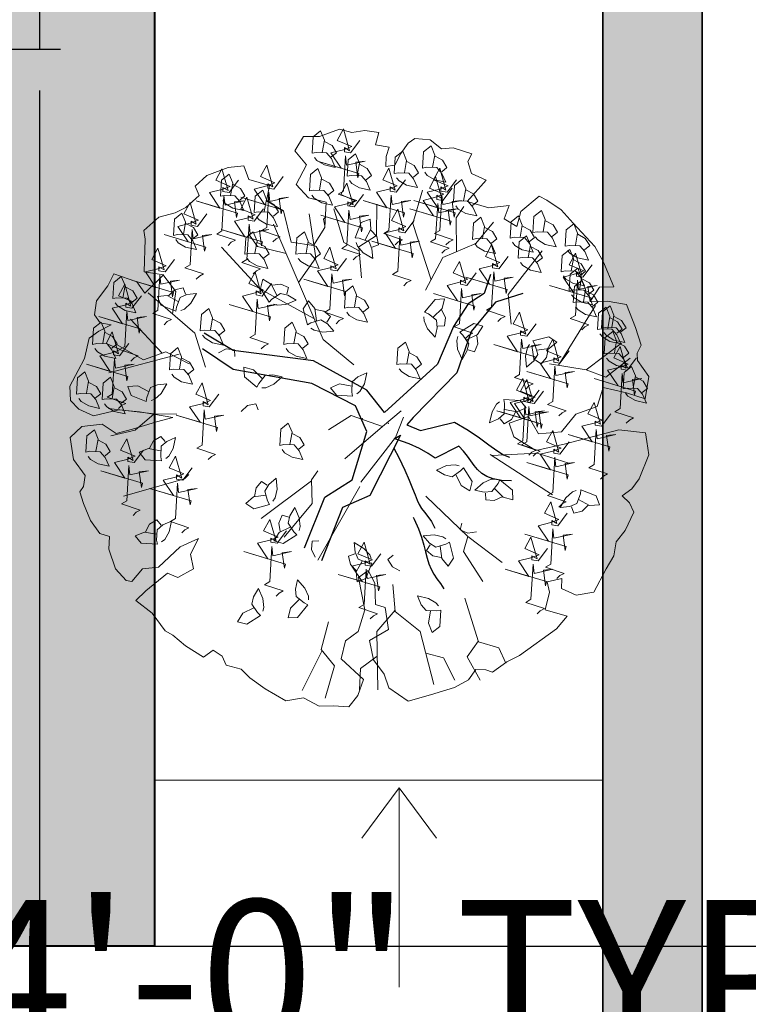
# Model space of a CAD drawing. Units: inches. Extents: x 2337 to 3570, y 1258 to 1938.
# Tile 25 of 30: x 3427 to 3471, y 1539 to 1598. Entities that reach past the tile are written whole.
import ezdxf

# ---------------------------------------------------------------- set-up
doc = ezdxf.new("R2010")
doc.units = ezdxf.units.IN
for name, color, linetype, lineweight in [('A-ANNO-DIMS', 2, 'Continuous', 18), ('A-ANNO-SYMB', 7, 'Continuous', 18), ('A-FLOR-STRS', 7, 'Continuous', 20), ('A-WALL', 7, 'Continuous', 40), ('ARBOL', 74, 'Continuous', 13), ('C-PROP', 7, 'Continuous', 35)]:
    doc.layers.add(name, color=color, linetype=linetype, lineweight=lineweight)
doc.layers.add('A-WALL-PATT', color=18, linetype='Continuous', lineweight=13, true_color=0x000000)
doc.layers.add('C-PROP-PATT', color=251, linetype='Continuous', lineweight=13, true_color=0x636466)
doc.layers.add('TALLO', color=36, linetype='Continuous')
doc.styles.get("Standard").update_dxf_attribs({"font": 'arial.ttf'})
doc.dimstyles.new('ISO-25', dxfattribs={"dimtxt": 9, "dimasz": 2.5, "dimexe": 1.25, "dimexo": 0.625, "dimtad": 1, "dimdec": 1, "dimlunit": 3, "dimtxsty": 'Standard', "dimcen": 2.5, "dimadec": 0, "dimazin": 0, "dimtfac": 1, "dimtdec": 1, "dimtmove": 0, "dimatfit": 3, "dimfxl": 1, "dimarcsym": 0})

# ---------------------------------------------------------------- blocks, each defined once
blk = doc.blocks.new('fresno')
at = {"layer": 'ARBOL'}
for p, q in [((2.96, 0.991), (3.575, 1.984)), ((-3.638, 1.194), (-4.164, 1.76)), ((-1.151, -0.932), (-1.99, -1.556)), ((-0.974, -3.757), (-1.31, -4.423))]:
    blk.add_line(p, q, dxfattribs=at)
blk.add_lwpolyline([(0.823, 4.745), (0.566, 4.764), (0.459, 4.687), (0.336, 4.518), (0.233, 4.322), (0.087, 4.298), (0.091, 4.464), (0.14, 4.621), (-0.09, 4.659), (-0.033, 4.863), (-0.264, 4.901), (-0.483, 4.866), (-0.686, 4.924), (-1.021, 4.801), (-1.288, 4.8), (-1.431, 4.563), (-1.234, 4.327), (-1.406, 4), (-1.205, 3.778), (-0.909, 3.705), (-0.931, 3.283), (-1.122, 2.983), (-1.491, 3.043), (-1.619, 3.562), (-1.9, 3.727), (-1.851, 3.982), (-2.197, 4.084), (-2.278, 4.31), (-2.543, 4.283), (-2.896, 4.152), (-3.091, 3.971), (-3.022, 3.817), (-3.244, 3.617), (-3.424, 3.528), (-3.697, 3.455), (-3.946, 3.236), (-3.922, 3.09), (-3.94, 2.548), (-3.617, 2.495), (-3.927, 2.19), (-4.062, 2.379), (-4.443, 2.512), (-4.546, 2.316), (-4.73, 2.062), (-4.767, 1.832), (-4.671, 1.698), (-4.486, 1.667), (-4.693, 1.559), (-4.854, 1.444), (-4.934, 1.102), (-5.037, 0.905), (-5.175, 0.644), (-5.166, 0.406), (-5.024, 0.264), (-4.781, 0.153), (-4.363, 0.249), (-4.014, 0.215), (-3.783, 0.177), (-3.46, 0.124), (-3.733, 0.051), (-4.132, -0.073), (-4.404, -0.146), (-4.639, 0.011), (-4.977, -0.028), (-5.172, -0.209), (-5.113, -0.574), (-4.921, -0.843), (-4.951, -1.027), (-5.012, -1.112), (-4.95, -1.311), (-4.83, -1.592), (-4.676, -1.807), (-4.518, -1.856), (-4.529, -2.068), (-4.417, -2.394), (-4.236, -2.59), (-4.143, -2.605), (-3.967, -2.397), (-3.703, -2.37), (-3.339, -2.027), (-3.032, -1.889), (-3.169, -2.15), (-3.115, -2.396), (-3.376, -2.542), (-3.552, -2.466), (-3.909, -2.762), (-4.077, -2.924), (-3.804, -3.135), (-3.592, -3.43), (-3.461, -3.499), (-3.253, -3.676), (-2.953, -3.867), (-2.792, -3.752), (-2.642, -3.848), (-2.572, -4.001), (-2.323, -4.066), (-2.18, -4.208), (-1.926, -4.392), (-1.58, -4.591), (-1.288, -4.545), (-1.027, -4.683), (-0.788, -4.675), (-0.531, -4.693), (-0.382, -4.505), (-0.29, -4.236), (-0.66, -3.891), (-0.588, -3.595), (-0.374, -3.441), (-0.267, -3.079), (-0.368, -2.541), (-0.208, -2.426), (-0.099, -2.633), (-0.087, -2.991), (0.071, -3.04), (0.129, -3.405), (-0.185, -3.59), (-0.119, -3.909), (0.055, -4.151), (0.136, -4.377), (0.456, -4.596), (0.828, -4.491), (1.227, -4.368), (1.461, -4.241), (1.583, -4.071), (1.748, -4.075), (1.86, -4.117), (2.101, -3.944), (2.308, -3.836), (2.925, -3.393), (3.101, -3.185), (2.74, -3.078), (2.812, -2.782), (2.769, -2.61), (3.015, -2.555), (3.012, -2.721), (3.254, -2.832), (3.546, -2.785), (3.752, -2.393), (3.882, -2.177), (3.92, -1.947), (4.069, -1.758), (4.214, -1.451), (4.144, -1.297), (4.021, -1.182), (4.182, -1.067), (4.304, -0.897), (4.464, -0.497), (4.429, -0.279), (4.406, -0.133), (3.964, -0.083), (3.074, -0.315), (2.582, -0.424), (2.217, -0.197), (2.136, 0.029), (2.462, 0.141), (2.628, -0.147), (3.012, -0.116), (3.249, 0.177), (3.602, 0.308), (3.701, 0.623), (4.089, 0.535), (4.404, 0.436), (4.464, 0.805), (4.272, 1.074), (4.267, 1.193), (4.336, 1.324), (4.243, 1.623), (4.092, 2.003), (3.769, 2.057), (3.485, 2.056), (3.642, 2.291), (3.88, 2.299), (3.71, 2.706), (3.563, 2.967), (3.201, 3.358), (3.001, 3.581), (2.766, 3.738), (2.635, 3.807), (2.332, 3.549), (2.268, 3.299), (2.052, 3.429), (2.136, 3.652), (1.798, 3.613), (1.437, 3.72), (1.755, 4.071), (1.513, 4.182), (1.451, 4.381), (1.519, 4.512), (1.204, 4.611), (1.012, 4.596)], close=True, dxfattribs=at)
for points in [[(-0.346, 4.735), (-0.501, 4.528), (-0.605, 4.545), (-0.605, 4.614), (-0.519, 4.563), (-0.622, 4.925), (-0.726, 4.735), (-0.484, 4.632), (-0.622, 4.58), (-0.829, 4.528), (-0.657, 4.27), (-1.053, 4.39), (-0.363, 4.183), (-0.381, 4.114), (-0.415, 4.373), (-0.26, 4.39), (-0.57, 4.321), (-0.588, 4.476), (-0.622, 3.89), (-0.708, 3.839), (-0.398, 3.735), (-0.467, 3.701), (-0.519, 3.649)], [(-1.104, 4.45), (-1.063, 4.399), (-0.939, 4.325), (-0.757, 4.285), (-0.82, 4.431), (-0.903, 4.527), (-1.075, 4.533), (-1.143, 4.521), (-1.126, 4.792), (-1.002, 4.891), (-0.939, 4.738), (-0.975, 4.535)], [(-0.935, 4.717), (-0.809, 4.65), (-0.736, 4.529), (-0.824, 4.459)], [(0.734, 4.203), (0.775, 4.152), (0.9, 4.078), (1.082, 4.038), (1.018, 4.185), (0.936, 4.281), (0.763, 4.287), (0.696, 4.274), (0.712, 4.546), (0.837, 4.645), (0.899, 4.491), (0.863, 4.289)], [(-0.521, 4.069), (-0.48, 4.018), (-0.356, 3.944), (-0.174, 3.904), (-0.237, 4.051), (-0.32, 4.146), (-0.492, 4.152), (-0.56, 4.14), (-0.543, 4.411), (-0.419, 4.511), (-0.356, 4.357), (-0.392, 4.154)], [(0.263, 4.114), (0.304, 4.063), (0.429, 3.989), (0.611, 3.948), (0.547, 4.095), (0.465, 4.191), (0.293, 4.197), (0.225, 4.185), (0.242, 4.456), (0.366, 4.555), (0.428, 4.402), (0.393, 4.199)], [(0.904, 4.471), (1.029, 4.404), (1.102, 4.282), (1.015, 4.212)], [(-2.368, 4.073), (-2.523, 3.866), (-2.627, 3.883), (-2.627, 3.952), (-2.541, 3.9), (-2.644, 4.262), (-2.748, 4.073), (-2.506, 3.969), (-2.644, 3.918), (-2.851, 3.866), (-2.679, 3.607), (-3.075, 3.728), (-2.385, 3.521), (-2.403, 3.452), (-2.437, 3.711), (-2.282, 3.728), (-2.592, 3.659), (-2.61, 3.814), (-2.644, 3.228), (-2.73, 3.176), (-2.42, 3.073), (-2.489, 3.038), (-2.541, 2.987)], [(-1.623, 4.132), (-1.778, 3.925), (-1.882, 3.942), (-1.882, 4.011), (-1.795, 3.959), (-1.899, 4.321), (-2.002, 4.132), (-1.761, 4.028), (-1.899, 3.977), (-2.106, 3.925), (-1.933, 3.666), (-2.33, 3.787), (-1.64, 3.58), (-1.657, 3.511), (-1.692, 3.77), (-1.537, 3.787), (-1.847, 3.718), (-1.864, 3.873), (-1.899, 3.287), (-1.985, 3.235), (-1.675, 3.132), (-1.744, 3.097), (-1.795, 3.046)], [(-1.149, 3.822), (-1.108, 3.771), (-0.983, 3.697), (-0.802, 3.657), (-0.865, 3.804), (-0.948, 3.9), (-1.12, 3.906), (-1.188, 3.893), (-1.171, 4.165), (-1.047, 4.264), (-0.984, 4.111), (-1.02, 3.908)], [(-0.352, 4.337), (-0.226, 4.269), (-0.153, 4.148), (-0.241, 4.078)], [(0.413, 4.08), (0.258, 3.873), (0.154, 3.89), (0.154, 3.959), (0.241, 3.908), (0.137, 4.27), (0.034, 4.08), (0.275, 3.977), (0.137, 3.925), (-0.07, 3.873), (0.103, 3.614), (-0.294, 3.735), (0.396, 3.528), (0.379, 3.459), (0.344, 3.718), (0.499, 3.735), (0.189, 3.666), (0.172, 3.821), (0.137, 3.235), (0.051, 3.183), (0.361, 3.08), (0.292, 3.046), (0.241, 2.994)], [(0.433, 4.381), (0.558, 4.314), (0.631, 4.193), (0.544, 4.122)], [(1.259, 4.08), (1.103, 3.873), (1, 3.89), (1, 3.959), (1.086, 3.908), (0.982, 4.27), (0.879, 4.08), (1.12, 3.977), (0.982, 3.925), (0.775, 3.873), (0.948, 3.614), (0.551, 3.735), (1.241, 3.528), (1.224, 3.459), (1.189, 3.718), (1.345, 3.735), (1.034, 3.666), (1.017, 3.821), (0.982, 3.235), (0.896, 3.183), (1.207, 3.08), (1.138, 3.046), (1.086, 2.994)], [(-2.629, 3.733), (-2.588, 3.682), (-2.463, 3.608), (-2.281, 3.568), (-2.345, 3.715), (-2.427, 3.81), (-2.6, 3.816), (-2.667, 3.804), (-2.651, 4.075), (-2.526, 4.175), (-2.464, 4.021), (-2.5, 3.818)], [(1.189, 3.942), (1.034, 3.735), (0.931, 3.752), (0.931, 3.821), (1.017, 3.77), (0.913, 4.132), (0.81, 3.942), (1.051, 3.839), (0.913, 3.787), (0.706, 3.735), (0.879, 3.477), (0.482, 3.597), (1.172, 3.39), (1.155, 3.321), (1.12, 3.58), (1.276, 3.597), (0.965, 3.528), (0.948, 3.683), (0.913, 3.097), (0.827, 3.046), (1.138, 2.942), (1.069, 2.908), (1.017, 2.856)], [(-2.459, 4), (-2.334, 3.933), (-2.261, 3.812), (-2.348, 3.742)], [(-0.287, 3.833), (-0.442, 3.626), (-0.546, 3.643), (-0.546, 3.712), (-0.46, 3.661), (-0.563, 4.023), (-0.667, 3.833), (-0.425, 3.73), (-0.563, 3.678), (-0.77, 3.626), (-0.598, 3.367), (-0.995, 3.488), (-0.304, 3.281), (-0.322, 3.212), (-0.356, 3.471), (-0.201, 3.488), (-0.511, 3.419), (-0.529, 3.574), (-0.563, 2.988), (-0.649, 2.936), (-0.339, 2.833), (-0.408, 2.799), (-0.46, 2.747)], [(-0.98, 4.09), (-0.854, 4.023), (-0.781, 3.901), (-0.869, 3.831)], [(1.25, 3.643), (1.291, 3.592), (1.416, 3.518), (1.597, 3.478), (1.534, 3.625), (1.451, 3.721), (1.279, 3.727), (1.211, 3.714), (1.228, 3.985), (1.352, 4.085), (1.415, 3.931), (1.379, 3.729)], [(-1.951, 3.597), (-2.106, 3.39), (-2.209, 3.408), (-2.209, 3.477), (-2.123, 3.425), (-2.227, 3.787), (-2.33, 3.597), (-2.089, 3.494), (-2.227, 3.442), (-2.434, 3.39), (-2.261, 3.132), (-2.658, 3.252), (-1.968, 3.046), (-1.985, 2.977), (-2.02, 3.235), (-1.864, 3.252), (-2.175, 3.183), (-2.192, 3.339), (-2.227, 2.752), (-2.313, 2.701), (-2.002, 2.597), (-2.071, 2.563), (-2.123, 2.511)], [(-2.068, 3.464), (-2.027, 3.413), (-1.903, 3.339), (-1.721, 3.299), (-1.784, 3.446), (-1.867, 3.542), (-2.039, 3.547), (-2.107, 3.535), (-2.09, 3.806), (-1.966, 3.906), (-1.903, 3.752), (-1.939, 3.55)], [(0.837, 2.414), (0.533, 3.352), (0.697, 3.906)], [(1.419, 3.911), (1.545, 3.844), (1.618, 3.722), (1.53, 3.652)], [(-2.898, 3.511), (-3.053, 3.304), (-3.157, 3.321), (-3.157, 3.39), (-3.071, 3.339), (-3.174, 3.701), (-3.278, 3.511), (-3.036, 3.408), (-3.174, 3.356), (-3.381, 3.304), (-3.209, 3.046), (-3.605, 3.166), (-2.915, 2.959), (-2.932, 2.89), (-2.967, 3.149), (-2.812, 3.166), (-3.122, 3.097), (-3.14, 3.253), (-3.174, 2.666), (-3.26, 2.615), (-2.95, 2.511), (-3.019, 2.477), (-3.071, 2.425)], [(-1.899, 3.732), (-1.773, 3.664), (-1.7, 3.543), (-1.788, 3.473)], [(-0.063, 3.671), (-0.069, 3.151), (-0.364, 2.965), (-0.319, 2.449)], [(1.259, 2.882), (1.254, 3.446), (1.381, 3.636)], [(-3.413, 3.083), (-3.373, 3.032), (-3.248, 2.958), (-3.066, 2.918), (-3.129, 3.065), (-3.212, 3.161), (-3.384, 3.167), (-3.452, 3.154), (-3.435, 3.425), (-3.311, 3.525), (-3.248, 3.371), (-3.284, 3.169)], [(-1.367, 2.367), (-1.081, 2.78), (-1.193, 3.514)], [(-0.923, 3.449), (-0.951, 3.425), (-0.93, 3.313)], [(-0.358, 2.895), (-0.615, 3.037), (-0.783, 3.596)], [(0.558, 3.402), (0.403, 3.195), (0.299, 3.212), (0.299, 3.281), (0.386, 3.23), (0.282, 3.592), (0.179, 3.402), (0.42, 3.299), (0.282, 3.247), (0.075, 3.195), (0.248, 2.936), (-0.149, 3.057), (0.541, 2.85), (0.524, 2.781), (0.489, 3.04), (0.644, 3.057), (0.334, 2.988), (0.317, 3.143), (0.282, 2.557), (0.196, 2.505), (0.506, 2.402), (0.437, 2.368), (0.386, 2.316)], [(1.564, 3.016), (1.605, 2.965), (1.729, 2.891), (1.911, 2.851), (1.848, 2.998), (1.765, 3.094), (1.593, 3.099), (1.525, 3.087), (1.542, 3.358), (1.666, 3.458), (1.729, 3.304), (1.693, 3.102)], [(2.191, 3.038), (2.232, 2.987), (2.357, 2.913), (2.539, 2.873), (2.475, 3.02), (2.393, 3.116), (2.221, 3.122), (2.153, 3.109), (2.17, 3.381), (2.294, 3.48), (2.356, 3.326), (2.321, 3.124)], [(2.573, 3.128), (2.613, 3.077), (2.738, 3.003), (2.92, 2.963), (2.857, 3.11), (2.774, 3.205), (2.602, 3.211), (2.534, 3.199), (2.551, 3.47), (2.675, 3.57), (2.738, 3.416), (2.702, 3.214)], [(-3.244, 3.351), (-3.118, 3.284), (-3.045, 3.162), (-3.133, 3.092)], [(-0.448, 1), (-0.961, 1.419), (-1.784, 3.341)], [(-0.41, 3.035), (-0.387, 2.974), (-0.291, 2.865), (-0.131, 2.771), (-0.146, 2.93), (-0.195, 3.047), (-0.357, 3.106), (-0.425, 3.115), (-0.325, 3.368), (-0.176, 3.424), (-0.164, 3.258), (-0.261, 3.077)], [(0.746, 2.242), (1.034, 2.786), (1.584, 3.019), (1.879, 3.374)], [(1.733, 3.284), (1.859, 3.216), (1.932, 3.095), (1.844, 3.025)], [(2.361, 3.306), (2.486, 3.239), (2.559, 3.117), (2.472, 3.047)], [(2.742, 3.396), (2.868, 3.328), (2.941, 3.207), (2.853, 3.137)], [(3.111, 2.904), (3.152, 2.853), (3.276, 2.779), (3.458, 2.739), (3.395, 2.886), (3.312, 2.981), (3.14, 2.987), (3.072, 2.975), (3.089, 3.246), (3.213, 3.346), (3.276, 3.192), (3.24, 2.99)], [(-2.225, 2.77), (-2.184, 2.718), (-2.06, 2.645), (-1.878, 2.604), (-1.941, 2.751), (-2.024, 2.847), (-2.196, 2.853), (-2.264, 2.84), (-2.247, 3.112), (-2.123, 3.211), (-2.06, 3.058), (-2.096, 2.855)], [(-1.575, 2.854), (-2.052, 2.969), (-2.2, 3.178)], [(-1.373, 2.77), (-1.332, 2.718), (-1.208, 2.645), (-1.026, 2.604), (-1.089, 2.751), (-1.172, 2.847), (-1.344, 2.853), (-1.412, 2.84), (-1.395, 3.112), (-1.271, 3.211), (-1.208, 3.058), (-1.244, 2.855)], [(-0.166, 3.238), (-0.068, 3.135), (-0.036, 2.997), (-0.141, 2.957)], [(2.326, 2.702), (2.367, 2.651), (2.492, 2.577), (2.673, 2.537), (2.61, 2.684), (2.527, 2.78), (2.355, 2.786), (2.287, 2.773), (2.304, 3.045), (2.428, 3.144), (2.491, 2.99), (2.455, 2.788)], [(3.28, 3.172), (3.406, 3.104), (3.479, 2.983), (3.391, 2.913)], [(-1.112, 1.773), (-2.014, 2.265), (-2.654, 2.957)], [(-2.056, 3.037), (-1.93, 2.97), (-1.857, 2.849), (-1.945, 2.778)], [(-0.57, 2.77), (-0.726, 2.563), (-0.829, 2.58), (-0.829, 2.649), (-0.743, 2.597), (-0.846, 2.959), (-0.95, 2.77), (-0.708, 2.666), (-0.846, 2.615), (-1.053, 2.563), (-0.881, 2.304), (-1.278, 2.425), (-0.588, 2.218), (-0.605, 2.149), (-0.639, 2.408), (-0.484, 2.425), (-0.795, 2.356), (-0.812, 2.511), (-0.846, 1.925), (-0.933, 1.873), (-0.622, 1.77), (-0.691, 1.735), (-0.743, 1.684)], [(-1.204, 3.037), (-1.078, 2.97), (-1.005, 2.849), (-1.093, 2.778)], [(2.121, 2.804), (1.966, 2.597), (1.862, 2.615), (1.862, 2.683), (1.949, 2.632), (1.845, 2.994), (1.742, 2.804), (1.983, 2.701), (1.845, 2.649), (1.638, 2.597), (1.811, 2.339), (1.414, 2.459), (2.104, 2.252), (2.087, 2.184), (2.052, 2.442), (2.207, 2.459), (1.897, 2.39), (1.88, 2.546), (1.845, 1.959), (1.759, 1.908), (2.069, 1.804), (2, 1.77), (1.949, 1.718)], [(2.495, 2.97), (2.621, 2.903), (2.694, 2.781), (2.606, 2.711)], [(-3.434, 2.752), (-3.59, 2.546), (-3.693, 2.563), (-3.693, 2.632), (-3.607, 2.58), (-3.71, 2.942), (-3.814, 2.752), (-3.572, 2.649), (-3.71, 2.597), (-3.917, 2.546), (-3.745, 2.287), (-4.142, 2.408), (-3.452, 2.201), (-3.469, 2.132), (-3.503, 2.39), (-3.348, 2.408), (-3.659, 2.339), (-3.676, 2.494), (-3.71, 1.908), (-3.797, 1.856), (-3.486, 1.753), (-3.555, 1.718), (-3.607, 1.666)], [(2.171, 1.674), (2.121, 2.172), (2.689, 2.898)], [(3.519, 2.666), (3.363, 2.459), (3.26, 2.477), (3.26, 2.546), (3.346, 2.494), (3.243, 2.856), (3.139, 2.666), (3.381, 2.563), (3.243, 2.511), (3.036, 2.459), (3.208, 2.201), (2.811, 2.321), (3.501, 2.115), (3.484, 2.046), (3.45, 2.304), (3.605, 2.321), (3.294, 2.252), (3.277, 2.408), (3.243, 1.821), (3.156, 1.77), (3.467, 1.666), (3.398, 1.632), (3.346, 1.58)], [(3.043, 2.478), (3.084, 2.427), (3.209, 2.353), (3.391, 2.313), (3.327, 2.46), (3.245, 2.556), (3.073, 2.562), (3.005, 2.549), (3.022, 2.82), (3.146, 2.92), (3.208, 2.766), (3.173, 2.564)], [(1.586, 2.528), (1.431, 2.321), (1.327, 2.339), (1.327, 2.408), (1.414, 2.356), (1.31, 2.718), (1.207, 2.528), (1.448, 2.425), (1.31, 2.373), (1.103, 2.321), (1.276, 2.063), (0.879, 2.184), (1.569, 1.977), (1.552, 1.908), (1.517, 2.166), (1.673, 2.184), (1.362, 2.115), (1.345, 2.27), (1.31, 1.684), (1.224, 1.632), (1.535, 1.528), (1.466, 1.494), (1.414, 1.442)], [(3.213, 2.746), (3.338, 2.679), (3.411, 2.557), (3.324, 2.487)], [(-4.422, 2.03), (-4.381, 1.979), (-4.257, 1.905), (-4.075, 1.865), (-4.138, 2.012), (-4.221, 2.108), (-4.393, 2.114), (-4.461, 2.101), (-4.444, 2.372), (-4.32, 2.472), (-4.257, 2.318), (-4.293, 2.116)], [(-3.468, 1.85), (-3.409, 2.222), (-3.628, 2.505)], [(-1.817, 2.351), (-1.972, 2.144), (-2.075, 2.162), (-2.075, 2.231), (-1.989, 2.179), (-2.093, 2.541), (-2.196, 2.351), (-1.955, 2.248), (-2.093, 2.196), (-2.3, 2.144), (-2.127, 1.886), (-2.524, 2.006), (-1.834, 1.8), (-1.851, 1.731), (-1.886, 1.989), (-1.73, 2.006), (-2.041, 1.937), (-2.058, 2.093), (-2.093, 1.506), (-2.179, 1.455), (-1.868, 1.351), (-1.937, 1.317), (-1.989, 1.265)], [(3.178, 2.165), (3.219, 2.113), (3.344, 2.04), (3.525, 1.999), (3.462, 2.146), (3.379, 2.242), (3.207, 2.248), (3.139, 2.236), (3.156, 2.507), (3.28, 2.606), (3.343, 2.453), (3.307, 2.25)], [(-3.986, 2.149), (-4.142, 1.942), (-4.245, 1.959), (-4.245, 2.028), (-4.159, 1.977), (-4.262, 2.339), (-4.366, 2.149), (-4.124, 2.046), (-4.262, 1.994), (-4.47, 1.942), (-4.297, 1.684), (-4.694, 1.804), (-4.004, 1.597), (-4.021, 1.528), (-4.055, 1.787), (-3.9, 1.804), (-4.211, 1.735), (-4.228, 1.89), (-4.262, 1.304), (-4.349, 1.253), (-4.038, 1.149), (-4.107, 1.115), (-4.159, 1.063)], [(-4.253, 2.298), (-4.127, 2.231), (-4.054, 2.109), (-4.142, 2.039)], [(-1.786, 2.007), (-1.722, 1.99), (-1.578, 2.003), (-1.407, 2.078), (-1.545, 2.159), (-1.668, 2.188), (-1.811, 2.092), (-1.859, 2.042), (-2.004, 2.271), (-1.962, 2.425), (-1.821, 2.337), (-1.731, 2.152)], [(-1.806, 2.323), (-1.665, 2.343), (-1.534, 2.287), (-1.564, 2.179)], [(-0.566, 1.873), (-0.525, 1.822), (-0.4, 1.748), (-0.219, 1.708), (-0.282, 1.855), (-0.365, 1.951), (-0.537, 1.957), (-0.605, 1.944), (-0.588, 2.216), (-0.464, 2.315), (-0.401, 2.162), (-0.437, 1.959)], [(3.245, 1.963), (3.286, 1.912), (3.411, 1.838), (3.593, 1.798), (3.529, 1.945), (3.447, 2.041), (3.274, 2.046), (3.206, 2.034), (3.223, 2.305), (3.347, 2.405), (3.41, 2.251), (3.374, 2.049)], [(3.347, 2.432), (3.473, 2.365), (3.546, 2.244), (3.458, 2.173)], [(-2.916, 0.958), (-3.096, 1.528), (-3.871, 2.197)], [(-3.331, 1.905), (-3.269, 1.928), (-3.161, 2.024), (-3.066, 2.184), (-3.226, 2.169), (-3.342, 2.121), (-3.401, 1.958), (-3.41, 1.89), (-3.663, 1.99), (-3.719, 2.139), (-3.554, 2.151), (-3.372, 2.054)], [(-3.533, 2.149), (-3.43, 2.247), (-3.292, 2.279), (-3.252, 2.174)], [(-0.397, 2.141), (-0.271, 2.074), (-0.198, 1.952), (-0.286, 1.882)], [(3.415, 2.231), (3.54, 2.163), (3.613, 2.042), (3.525, 1.972)], [(-1.164, 1.612), (-1.109, 1.576), (-0.967, 1.544), (-0.782, 1.562), (-0.888, 1.682), (-0.996, 1.748), (-1.162, 1.7), (-1.222, 1.667), (-1.29, 1.93), (-1.203, 2.063), (-1.096, 1.937), (-1.067, 1.733)], [(0.72, 1.798), (0.723, 1.733), (0.781, 1.6), (0.904, 1.46), (0.939, 1.616), (0.929, 1.742), (0.793, 1.848), (0.73, 1.878), (0.904, 2.088), (1.062, 2.095), (1.023, 1.934), (0.875, 1.791)], [(3.716, 1.537), (3.757, 1.486), (3.882, 1.412), (4.063, 1.372), (4, 1.519), (3.917, 1.615), (3.745, 1.621), (3.677, 1.608), (3.694, 1.88), (3.818, 1.979), (3.881, 1.825), (3.845, 1.623)], [(-2.965, 1.493), (-2.924, 1.441), (-2.799, 1.368), (-2.618, 1.327), (-2.681, 1.474), (-2.764, 1.57), (-2.936, 1.576), (-3.004, 1.564), (-2.987, 1.835), (-2.863, 1.934), (-2.8, 1.781), (-2.836, 1.578)], [(-1.085, 1.919), (-0.945, 1.893), (-0.838, 1.801), (-0.9, 1.707)], [(1.014, 1.915), (1.077, 1.787), (1.064, 1.646), (0.952, 1.64)], [(2.587, 1.684), (2.432, 1.477), (2.328, 1.494), (2.328, 1.563), (2.414, 1.511), (2.311, 1.873), (2.207, 1.684), (2.449, 1.58), (2.311, 1.528), (2.104, 1.477), (2.276, 1.218), (1.88, 1.339), (2.57, 1.132), (2.552, 1.063), (2.518, 1.321), (2.673, 1.339), (2.363, 1.27), (2.345, 1.425), (2.311, 0.839), (2.225, 0.787), (2.535, 0.684), (2.466, 0.649), (2.414, 0.597)], [(3.649, 1.515), (3.69, 1.464), (3.814, 1.39), (3.996, 1.35), (3.933, 1.497), (3.85, 1.592), (3.678, 1.598), (3.61, 1.586), (3.627, 1.857), (3.751, 1.957), (3.814, 1.803), (3.778, 1.601)], [(3.885, 1.805), (4.011, 1.738), (4.084, 1.616), (3.996, 1.546)], [(-4.759, 1.269), (-4.718, 1.217), (-4.593, 1.144), (-4.411, 1.103), (-4.475, 1.25), (-4.557, 1.346), (-4.729, 1.352), (-4.797, 1.339), (-4.78, 1.611), (-4.656, 1.71), (-4.594, 1.557), (-4.629, 1.354)], [(-2.796, 1.76), (-2.67, 1.693), (-2.597, 1.572), (-2.685, 1.501)], [(-1.575, 1.269), (-1.534, 1.217), (-1.409, 1.144), (-1.228, 1.103), (-1.291, 1.25), (-1.373, 1.346), (-1.546, 1.352), (-1.614, 1.339), (-1.597, 1.611), (-1.473, 1.71), (-1.41, 1.557), (-1.446, 1.354)], [(1.283, 1.469), (1.266, 1.405), (1.279, 1.261), (1.354, 1.09), (1.435, 1.228), (1.464, 1.351), (1.368, 1.494), (1.318, 1.542), (1.547, 1.687), (1.7, 1.645), (1.613, 1.504), (1.428, 1.414)], [(3.818, 1.783), (3.944, 1.715), (4.017, 1.594), (3.929, 1.524)], [(-4.193, 1.356), (-4.349, 1.149), (-4.452, 1.166), (-4.452, 1.235), (-4.366, 1.184), (-4.469, 1.546), (-4.573, 1.356), (-4.331, 1.253), (-4.469, 1.201), (-4.677, 1.149), (-4.504, 0.89), (-4.901, 1.011), (-4.211, 0.804), (-4.228, 0.735), (-4.262, 0.994), (-4.107, 1.011), (-4.418, 0.942), (-4.435, 1.097), (-4.469, 0.511), (-4.556, 0.459), (-4.245, 0.356), (-4.314, 0.322), (-4.366, 0.27)], [(-4.589, 1.536), (-4.464, 1.469), (-4.391, 1.348), (-4.478, 1.277)], [(-1.406, 1.536), (-1.28, 1.469), (-1.207, 1.348), (-1.295, 1.277)], [(1.599, 1.489), (1.618, 1.348), (1.563, 1.217), (1.455, 1.247)], [(3.761, 1.112), (3.802, 1.061), (3.926, 0.987), (4.108, 0.947), (4.045, 1.093), (3.962, 1.189), (3.79, 1.195), (3.722, 1.183), (3.739, 1.454), (3.863, 1.553), (3.926, 1.4), (3.89, 1.197)], [(-3.192, 1.017), (-3.578, 1.215), (-3.949, 1.081), (-4.398, 1.339)], [(0.308, 0.933), (0.349, 0.881), (0.474, 0.807), (0.656, 0.767), (0.592, 0.914), (0.51, 1.01), (0.337, 1.016), (0.27, 1.003), (0.286, 1.275), (0.411, 1.374), (0.473, 1.221), (0.437, 1.018)], [(2.479, 1.34), (2.443, 1.285), (2.411, 1.143), (2.429, 0.958), (2.549, 1.064), (2.615, 1.172), (2.567, 1.338), (2.534, 1.398), (2.797, 1.466), (2.93, 1.379), (2.804, 1.272), (2.6, 1.243)], [(3.139, 1.235), (2.984, 1.028), (2.88, 1.046), (2.88, 1.115), (2.967, 1.063), (2.863, 1.425), (2.759, 1.235), (3.001, 1.132), (2.863, 1.08), (2.656, 1.028), (2.828, 0.77), (2.432, 0.891), (3.122, 0.684), (3.105, 0.615), (3.07, 0.873), (3.225, 0.891), (2.915, 0.822), (2.897, 0.977), (2.863, 0.391), (2.777, 0.339), (3.087, 0.235), (3.018, 0.201), (2.967, 0.149)], [(4.01, 1.36), (3.422, 0.918)], [(3.93, 1.379), (4.056, 1.312), (4.129, 1.191), (4.041, 1.121)], [(-3.354, 1.176), (-4.529, 0.864)], [(-3.481, 0.843), (-3.44, 0.792), (-3.315, 0.718), (-3.133, 0.678), (-3.197, 0.825), (-3.279, 0.92), (-3.451, 0.926), (-3.519, 0.914), (-3.502, 1.185), (-3.378, 1.285), (-3.316, 1.131), (-3.351, 0.928)], [(-2.703, 1.201), (-2.575, 1.263), (-2.433, 1.251), (-2.428, 1.139)], [(0.478, 1.2), (0.603, 1.133), (0.676, 1.011), (0.589, 0.941)], [(2.786, 1.261), (2.76, 1.121), (2.668, 1.014), (2.574, 1.076)], [(4.26, 1.115), (4.105, 0.908), (4.002, 0.925), (4.002, 0.994), (4.088, 0.942), (3.984, 1.304), (3.881, 1.115), (4.122, 1.011), (3.984, 0.959), (3.777, 0.908), (3.95, 0.649), (3.553, 0.77), (4.243, 0.563), (4.226, 0.494), (4.191, 0.753), (4.347, 0.77), (4.036, 0.701), (4.019, 0.856), (3.984, 0.27), (3.898, 0.218), (4.209, 0.115), (4.14, 0.08), (4.088, 0.029)], [(-3.311, 1.111), (-3.186, 1.043), (-3.113, 0.922), (-3.2, 0.852)], [(2.808, 1.015), (3.422, 0.918), (3.422, 0.918), (3.748, 0.794), (4.154, 1.111)], [(-5.028, 0.44), (-4.987, 0.388), (-4.862, 0.315), (-4.68, 0.274), (-4.744, 0.421), (-4.826, 0.517), (-4.998, 0.523), (-5.066, 0.511), (-5.049, 0.782), (-4.925, 0.881), (-4.863, 0.728), (-4.898, 0.525)], [(-1.981, 0.615), (-1.915, 0.618), (-1.782, 0.676), (-1.643, 0.799), (-1.799, 0.834), (-1.925, 0.824), (-2.031, 0.688), (-2.061, 0.626), (-2.27, 0.799), (-2.278, 0.958), (-2.117, 0.918), (-1.974, 0.77)], [(-0.397, 0.517), (-0.346, 0.557), (-0.272, 0.682), (-0.232, 0.864), (-0.379, 0.801), (-0.474, 0.718), (-0.48, 0.546), (-0.468, 0.478), (-0.739, 0.495), (-0.838, 0.619), (-0.685, 0.682), (-0.482, 0.646)], [(4.075, 0.529), (4.116, 0.478), (4.24, 0.404), (4.422, 0.364), (4.359, 0.511), (4.276, 0.607), (4.104, 0.613), (4.036, 0.6), (4.053, 0.871), (4.177, 0.971), (4.24, 0.817), (4.204, 0.615)], [(-4.858, 0.707), (-4.733, 0.64), (-4.66, 0.519), (-4.747, 0.448)], [(-4.602, 0.35), (-4.561, 0.299), (-4.436, 0.225), (-4.254, 0.185), (-4.318, 0.332), (-4.4, 0.428), (-4.572, 0.433), (-4.64, 0.421), (-4.623, 0.692), (-4.499, 0.792), (-4.437, 0.638), (-4.472, 0.436)], [(-3.824, 0.404), (-3.763, 0.427), (-3.654, 0.523), (-3.559, 0.683), (-3.719, 0.668), (-3.835, 0.62), (-3.894, 0.457), (-3.903, 0.389), (-4.156, 0.489), (-4.212, 0.638), (-4.047, 0.65), (-3.865, 0.553)], [(-2.698, 0.509), (-2.854, 0.302), (-2.957, 0.319), (-2.957, 0.388), (-2.871, 0.336), (-2.974, 0.698), (-3.078, 0.509), (-2.836, 0.405), (-2.974, 0.353), (-3.182, 0.302), (-3.009, 0.043), (-3.406, 0.164), (-2.716, -0.043), (-2.733, -0.112), (-2.767, 0.147), (-2.612, 0.164), (-2.923, 0.095), (-2.94, 0.25), (-2.974, -0.336), (-3.061, -0.388), (-2.75, -0.491), (-2.819, -0.526), (-2.871, -0.577)], [(2.639, 0.58), (2.483, 0.373), (2.38, 0.391), (2.38, 0.46), (2.466, 0.408), (2.363, 0.77), (2.259, 0.58), (2.501, 0.477), (2.363, 0.425), (2.156, 0.373), (2.328, 0.115), (1.931, 0.235), (2.621, 0.029), (2.604, -0.04), (2.57, 0.218), (2.725, 0.235), (2.414, 0.166), (2.397, 0.322), (2.363, -0.265), (2.276, -0.316), (2.587, -0.42), (2.518, -0.454), (2.466, -0.506)], [(2.708, 0.563), (2.552, 0.356), (2.449, 0.373), (2.449, 0.442), (2.535, 0.391), (2.432, 0.753), (2.328, 0.563), (2.57, 0.46), (2.432, 0.408), (2.225, 0.356), (2.397, 0.097), (2, 0.218), (2.69, 0.011), (2.673, -0.058), (2.639, 0.201), (2.794, 0.218), (2.483, 0.149), (2.466, 0.304), (2.432, -0.282), (2.345, -0.334), (2.656, -0.437), (2.587, -0.471), (2.535, -0.523)], [(4.244, 0.797), (4.37, 0.73), (4.443, 0.608), (4.355, 0.538)], [(-4.432, 0.618), (-4.307, 0.55), (-4.234, 0.429), (-4.321, 0.359)], [(-2.322, 0.222), (-2.219, 0.321), (-2.081, 0.353), (-2.042, 0.248)], [(1.978, 0.384), (1.927, 0.343), (1.853, 0.218), (1.813, 0.036), (1.96, 0.1), (2.056, 0.182), (2.061, 0.355), (2.049, 0.422), (2.32, 0.406), (2.42, 0.281), (2.266, 0.219), (2.064, 0.254)], [(3.829, 0.184), (3.674, -0.023), (3.57, -0.006), (3.57, 0.063), (3.657, 0.011), (3.553, 0.373), (3.45, 0.184), (3.691, 0.08), (3.553, 0.029), (3.346, -0.023), (3.519, -0.282), (3.122, -0.161), (3.812, -0.368), (3.795, -0.437), (3.76, -0.178), (3.915, -0.161), (3.605, -0.23), (3.588, -0.075), (3.553, -0.661), (3.467, -0.713), (3.777, -0.816), (3.708, -0.851), (3.657, -0.902)], [(-3.394, 0.18), (-3.77, 0.182), (-4.532, 0.27)], [(-3.77, 0.182), (-4.09, -0.088), (-4.494, -0.18)], [(-0.596, -0.564), (0.03, -0.026), (0.339, 0.235)], [(2.246, 0.214), (2.178, 0.089), (2.057, 0.016), (1.987, 0.103)], [(-1.642, -0.412), (-1.601, -0.463), (-1.477, -0.537), (-1.295, -0.577), (-1.358, -0.43), (-1.441, -0.334), (-1.613, -0.328), (-1.681, -0.341), (-1.664, -0.069), (-1.54, 0.03), (-1.477, -0.124), (-1.513, -0.326)], [(0.03, -0.026), (-0.491, 0.154), (-0.871, -0.08)], [(0.38, 0.131), (0.248, -0.21), (-0.33, -0.951)], [(-4.871, -0.524), (-4.83, -0.575), (-4.705, -0.649), (-4.523, -0.689), (-4.587, -0.542), (-4.669, -0.446), (-4.841, -0.44), (-4.909, -0.453), (-4.893, -0.181), (-4.768, -0.082), (-4.706, -0.236), (-4.741, -0.438)], [(-1.473, -0.144), (-1.347, -0.211), (-1.274, -0.333), (-1.362, -0.403)], [(3.139, -0.282), (2.984, -0.489), (2.88, -0.471), (2.88, -0.402), (2.967, -0.454), (2.863, -0.092), (2.759, -0.282), (3.001, -0.385), (2.863, -0.437), (2.656, -0.489), (2.828, -0.747), (2.432, -0.627), (3.122, -0.834), (3.105, -0.902), (3.07, -0.644), (3.225, -0.627), (2.915, -0.696), (2.897, -0.54), (2.863, -1.127), (2.777, -1.178), (3.087, -1.282), (3.018, -1.316), (2.967, -1.368)], [(-4.701, -0.256), (-4.576, -0.323), (-4.503, -0.445), (-4.59, -0.515)], [(-3.952, -0.42), (-4.107, -0.627), (-4.211, -0.609), (-4.211, -0.54), (-4.124, -0.592), (-4.228, -0.23), (-4.331, -0.42), (-4.09, -0.523), (-4.228, -0.575), (-4.435, -0.627), (-4.262, -0.885), (-4.659, -0.765), (-3.969, -0.971), (-3.986, -1.04), (-4.021, -0.782), (-3.866, -0.765), (-4.176, -0.834), (-4.193, -0.678), (-4.228, -1.265), (-4.314, -1.316), (-4.004, -1.42), (-4.073, -1.454), (-4.124, -1.506)], [(-3.58, -0.559), (-3.529, -0.518), (-3.455, -0.393), (-3.415, -0.211), (-3.562, -0.275), (-3.658, -0.357), (-3.664, -0.53), (-3.651, -0.597), (-3.923, -0.581), (-4.022, -0.456), (-3.868, -0.394), (-3.666, -0.43)], [(-3.848, -0.389), (-3.781, -0.264), (-3.659, -0.191), (-3.589, -0.278)], [(1.846, -0.51), (2.605, -0.469), (3.129, -0.637)], [(-3.141, -0.713), (-3.296, -0.92), (-3.4, -0.902), (-3.4, -0.834), (-3.314, -0.885), (-3.417, -0.523), (-3.521, -0.713), (-3.279, -0.816), (-3.417, -0.868), (-3.624, -0.92), (-3.452, -1.178), (-3.848, -1.058), (-3.158, -1.265), (-3.175, -1.333), (-3.21, -1.075), (-3.055, -1.058), (-3.365, -1.127), (-3.383, -0.971), (-3.417, -1.558), (-3.503, -1.609), (-3.193, -1.713), (-3.262, -1.747), (-3.314, -1.799)], [(1.822, -0.495), (2.859, -1.165)], [(-1.047, -0.767), (-1.151, -0.913), (-1.144, -1.307), (-1.61, -1.871)], [(1.304, -0.681), (1.241, -0.664), (1.097, -0.678), (0.926, -0.752), (1.064, -0.833), (1.187, -0.862), (1.33, -0.766), (1.377, -0.716), (1.523, -0.945), (1.481, -1.099), (1.34, -1.011), (1.25, -0.826)], [(-3.195, -0.824), (-3.267, -0.898), (-4.285, -1.185)], [(-1.794, -1.268), (-1.758, -1.214), (-1.726, -1.072), (-1.744, -0.887), (-1.865, -0.993), (-1.93, -1.101), (-1.883, -1.266), (-1.85, -1.327), (-2.113, -1.395), (-2.246, -1.307), (-2.119, -1.2), (-1.916, -1.172)], [(-2.101, -1.19), (-2.076, -1.05), (-1.983, -0.943), (-1.889, -1.004)], [(1.903, -0.903), (1.837, -0.905), (1.704, -0.963), (1.565, -1.086), (1.721, -1.122), (1.847, -1.111), (1.953, -0.975), (1.983, -0.913), (2.192, -1.086), (2.2, -1.245), (2.039, -1.205), (1.896, -1.057)], [(-0.346, -1.024), (-1.05, -2.251)], [(2.02, -1.197), (1.891, -1.259), (1.75, -1.247), (1.745, -1.134)], [(3.253, -1.094), (3.192, -1.117), (3.083, -1.213), (2.988, -1.374), (3.148, -1.359), (3.264, -1.31), (3.323, -1.148), (3.332, -1.079), (3.585, -1.179), (3.641, -1.328), (3.476, -1.34), (3.294, -1.244)], [(0.748, -1.185), (1.452, -1.855), (2.021, -2.292)], [(3.105, -1.471), (2.949, -1.678), (2.846, -1.661), (2.846, -1.592), (2.932, -1.644), (2.829, -1.282), (2.725, -1.471), (2.967, -1.575), (2.829, -1.627), (2.621, -1.678), (2.794, -1.937), (2.397, -1.816), (3.087, -2.023), (3.07, -2.092), (3.036, -1.833), (3.191, -1.816), (2.88, -1.885), (2.863, -1.73), (2.829, -2.316), (2.742, -2.368), (3.053, -2.471), (2.984, -2.506), (2.932, -2.558)], [(-1.361, -1.756), (-1.343, -1.693), (-1.357, -1.548), (-1.431, -1.377), (-1.513, -1.515), (-1.542, -1.638), (-1.445, -1.781), (-1.395, -1.829), (-1.625, -1.974), (-1.778, -1.932), (-1.691, -1.791), (-1.506, -1.701)], [(3.455, -1.338), (3.352, -1.437), (3.214, -1.469), (3.175, -1.364)], [(-3.648, -1.948), (-3.596, -1.907), (-3.523, -1.782), (-3.482, -1.6), (-3.629, -1.664), (-3.725, -1.746), (-3.731, -1.919), (-3.719, -1.986), (-3.99, -1.97), (-4.089, -1.845), (-3.936, -1.783), (-3.733, -1.819)], [(-3.915, -1.778), (-3.848, -1.653), (-3.727, -1.58), (-3.656, -1.667)], [(-1.571, -1.764), (-1.726, -1.971), (-1.83, -1.954), (-1.83, -1.885), (-1.744, -1.937), (-1.847, -1.575), (-1.951, -1.764), (-1.709, -1.868), (-1.847, -1.92), (-2.054, -1.971), (-1.882, -2.23), (-2.278, -2.109), (-1.588, -2.316), (-1.605, -2.385), (-1.64, -2.127), (-1.485, -2.109), (-1.795, -2.178), (-1.813, -2.023), (-1.847, -2.609), (-1.933, -2.661), (-1.623, -2.764), (-1.692, -2.799), (-1.744, -2.851)], [(-1.677, -1.776), (-1.696, -1.635), (-1.641, -1.504), (-1.533, -1.534)], [(1.593, -1.781), (1.452, -1.801), (1.322, -1.746), (1.352, -1.637)], [(-1.092, -2.202), (-1.154, -2.074), (-1.142, -1.933), (-1.03, -1.928)], [(-0.001, -2.144), (-0.156, -2.351), (-0.26, -2.333), (-0.26, -2.264), (-0.174, -2.316), (-0.277, -1.954), (-0.381, -2.144), (-0.139, -2.247), (-0.277, -2.299), (-0.484, -2.351), (-0.312, -2.609), (-0.708, -2.489), (-0.018, -2.695), (-0.035, -2.764), (-0.07, -2.506), (0.085, -2.489), (-0.225, -2.558), (-0.243, -2.402), (-0.277, -2.989), (-0.363, -3.04), (-0.053, -3.144), (-0.122, -3.178), (-0.174, -3.23)], [(-0.161, -2.225), (-0.184, -2.163), (-0.28, -2.055), (-0.44, -1.96), (-0.425, -2.12), (-0.376, -2.236), (-0.214, -2.295), (-0.146, -2.304), (-0.246, -2.557), (-0.395, -2.613), (-0.407, -2.448), (-0.31, -2.266)], [(1.086, -1.899), (1.031, -1.863), (0.89, -1.831), (0.704, -1.849), (0.81, -1.969), (0.918, -2.035), (1.084, -1.987), (1.145, -1.954), (1.212, -2.218), (1.125, -2.35), (1.018, -2.224), (0.989, -2.02)], [(1.452, -1.855), (1.379, -2.105), (1.698, -2.609)], [(2.777, -2.058), (2.621, -2.264), (2.518, -2.247), (2.518, -2.178), (2.604, -2.23), (2.501, -1.868), (2.397, -2.058), (2.639, -2.161), (2.501, -2.213), (2.294, -2.264), (2.466, -2.523), (2.069, -2.402), (2.759, -2.609), (2.742, -2.678), (2.708, -2.42), (2.863, -2.402), (2.552, -2.471), (2.535, -2.316), (2.501, -2.902), (2.414, -2.954), (2.725, -3.057), (2.656, -3.092), (2.604, -3.144)], [(1.007, -2.206), (0.867, -2.181), (0.76, -2.088), (0.822, -1.994)], [(-0.405, -2.427), (-0.503, -2.324), (-0.535, -2.186), (-0.43, -2.146)], [(0.319, -2.428), (0.193, -2.361), (0.12, -2.239), (0.208, -2.169)], [(-1.201, -2.914), (-1.204, -2.849), (-1.262, -2.716), (-1.385, -2.576), (-1.42, -2.732), (-1.41, -2.858), (-1.274, -2.964), (-1.212, -2.994), (-1.385, -3.204), (-1.544, -3.211), (-1.504, -3.05), (-1.356, -2.907)], [(-1.966, -3.1), (-1.949, -3.037), (-1.962, -2.892), (-2.037, -2.722), (-2.118, -2.859), (-2.147, -2.982), (-2.051, -3.125), (-2.001, -3.173), (-2.23, -3.319), (-2.383, -3.277), (-2.296, -3.136), (-2.111, -3.046)], [(0.201, -2.655), (0.24, -3.105), (0.657, -3.436), (0.886, -4.322)], [(0.959, -3.012), (0.918, -2.961), (0.793, -2.887), (0.612, -2.847), (0.675, -2.994), (0.758, -3.089), (0.93, -3.095), (0.998, -3.083), (0.981, -3.354), (0.857, -3.453), (0.794, -3.3), (0.83, -3.097)], [(1.399, -2.886), (1.63, -3.612), (1.964, -3.708), (2.084, -3.964)], [(0.238, -3.084), (-0.067, -3.438), (-0.048, -4.412)], [(-0.923, -4.549), (-0.768, -4.012), (-0.99, -3.737), (-0.872, -3.28)], [(1.625, -3.596), (1.438, -3.858), (1.657, -4.248)], [(-0.059, -3.851), (-0.336, -4.054), (-0.355, -4.41)], [(0.752, -3.801), (1.042, -3.878), (1.233, -4.25)]]:
    blk.add_lwpolyline(points, dxfattribs=at)
for p in [(-0.308, 0.101), (0.124, 0.027)]:
    blk.add_point(p, dxfattribs=at)
at = {"layer": 'TALLO'}
for points in [[(1.829, 2.5), (1.722, 2.184), (1.454, 2.012), (1.213, 1.639), (0.944, 1.008), (0.06, 0.204), (-0.234, 0.577), (-1.119, 1.065), (-2.458, 1.237), (-2.941, 1.524)], [(2.364, 2.184), (1.909, 2.041), (1.507, 1.552), (1.266, 0.864), (0.542, 0.125), (0.433, 0.001), (0.662, -0.096), (1.228, 0.045), (1.455, -0.09), (1.644, -0.216), (1.8, -0.33), (1.931, -0.425), (2.042, -0.496), (2.141, -0.539)], [(-1.272, -2.047), (-0.931, -1.203), (-0.475, -0.916), (-0.234, -0.112), (-0.422, 0.318), (-1.146, 0.691), (-2.458, 0.921), (-2.967, 1.266)], [(2.177, -0.932), (2.008, -0.924), (1.873, -0.898), (1.766, -0.859), (1.682, -0.807), (1.613, -0.745), (1.554, -0.676), (1.499, -0.6), (1.442, -0.521), (1.376, -0.44), (1.298, -0.357), (0.908, -0.555), (0.791, -0.474), (0.647, -0.394), (0.474, -0.317), (0.265, -0.244), (0.226, -0.233), (0.328, -0.17), (-0.181, -1.175), (-0.637, -1.375), (-0.985, -2.265)], [(0.219, -0.386), (0.3, -0.544), (0.399, -0.753), (0.473, -0.922), (0.529, -1.057), (0.571, -1.164), (0.607, -1.251), (0.641, -1.324), (0.68, -1.389), (0.729, -1.454), (0.784, -1.525), (0.844, -1.61), (0.903, -1.717)], [(0.538, -1.536), (0.555, -1.568), (0.626, -1.728), (0.678, -1.871), (0.716, -2), (0.747, -2.115), (0.773, -2.219), (0.802, -2.314), (0.837, -2.401), (0.883, -2.483), (0.936, -2.562), (0.994, -2.642), (1.052, -2.727)]]:
    blk.add_lwpolyline(points, dxfattribs=at)
blk = doc.blocks.new('STAIR-UP-ARROW')
for p, q in [((2.25, 12), (2.25, 0)), ((2.25, 0), (0, 3.013)), ((2.25, 0), (4.5, 3.013))]:
    blk.add_line(p, q)
blk = doc.blocks.new('*D68')
at = {"layer": 'A-ANNO-DIMS', "color": 0, "lineweight": -2, "transparency": 16777216}
for p, q in [((3427.886, 1596.116), (3427.886, 1741.994)), ((3420.411, 1596.116), (3429.136, 1596.116)), ((3427.886, 1544.616), (3427.886, 1593.616)), ((3420.411, 1542.116), (3429.136, 1542.116))]:
    blk.add_line(p, q, dxfattribs=at)
at = {"layer": 'A-ANNO-DIMS', "color": 0, "transparency": 16777216}
for points in [[(3427.469, 1593.616), (3428.303, 1593.616), (3427.886, 1596.116)], [(3427.469, 1544.616), (3428.303, 1544.616), (3427.886, 1542.116)]]:
    blk.add_solid(points, dxfattribs=at)
at = {"layer": 'Defpoints', "color": 0, "transparency": 16777216}
for p in [(3419.786, 1596.116), (3427.886, 1596.116), (3419.786, 1542.116)]:
    blk.add_point(p, dxfattribs=at)
at = {"layer": 'A-ANNO-DIMS', "color": 0, "transparency": 16777216, "insert": (3422.605, 1670.305), "char_height": 9, "attachment_point": 5, "rotation": 90}
blk.add_mtext('SWING DOOR 4\'-6" TYP.', dxfattribs=at)
blk = doc.blocks.new('*D69')
at = {"layer": 'A-ANNO-DIMS', "color": 0, "lineweight": -2, "transparency": 16777216}
for p, q in [((3371.786, 1541.491), (3371.786, 1532.766)), ((3419.786, 1541.491), (3419.786, 1532.766)), ((3374.286, 1534.016), (3417.286, 1534.016)), ((3419.786, 1534.016), (3478.758, 1534.016))]:
    blk.add_line(p, q, dxfattribs=at)
at = {"layer": 'A-ANNO-DIMS', "color": 0, "transparency": 16777216}
for points in [[(3374.286, 1534.433), (3374.286, 1533.599), (3371.786, 1534.016)], [(3417.286, 1534.433), (3417.286, 1533.599), (3419.786, 1534.016)]]:
    blk.add_solid(points, dxfattribs=at)
at = {"layer": 'Defpoints', "color": 0, "transparency": 16777216}
for p in [(3371.786, 1542.116), (3419.786, 1542.116), (3419.786, 1534.016)]:
    blk.add_point(p, dxfattribs=at)
at = {"layer": 'A-ANNO-DIMS', "color": 0, "transparency": 16777216, "insert": (3450.522, 1539.236), "char_height": 9, "attachment_point": 5}
blk.add_mtext('4\'-0" TYP.', dxfattribs=at)
blk = doc.blocks.new('*D115')
at = {"layer": 'A-ANNO-DIMS', "color": 0, "lineweight": -2, "transparency": 16777216}
for p, q in [((3243.411, 1542.116), (3502.436, 1542.116)), ((3501.186, 1539.616), (3501.186, 1526.616)), ((3243.411, 1524.116), (3502.436, 1524.116)), ((3501.186, 1524.116), (3501.186, 1497.289))]:
    blk.add_line(p, q, dxfattribs=at)
at = {"layer": 'A-ANNO-DIMS', "color": 0, "transparency": 16777216}
for points in [[(3500.769, 1539.616), (3501.603, 1539.616), (3501.186, 1542.116)], [(3500.769, 1526.616), (3501.603, 1526.616), (3501.186, 1524.116)]]:
    blk.add_solid(points, dxfattribs=at)
at = {"layer": 'Defpoints', "color": 0, "transparency": 16777216}
for p in [(3242.786, 1542.116), (3242.786, 1524.116), (3501.186, 1524.116)]:
    blk.add_point(p, dxfattribs=at)
at = {"layer": 'A-ANNO-DIMS', "color": 0, "transparency": 16777216, "insert": (3495.966, 1509.452), "char_height": 9, "attachment_point": 5, "rotation": 90}
blk.add_mtext('1\'-6"', dxfattribs=at)

msp = doc.modelspace()

# ---------------------------------------------------------------- hatches: boundary and pattern name
at = {"layer": 'A-WALL-PATT'}
h = msp.add_hatch(color=256, dxfattribs=at)
h.dxf.hatch_style = 1
h.paths.add_polyline_path([(3233.786, 1857.116), (3017.786, 1857.116), (3017.786, 1824.116), (3026.786, 1824.116), (3026.786, 1848.116), (3233.786, 1848.116)])
h.paths.add_polyline_path([(3128.786, 1764.116), (3026.786, 1764.116), (3026.786, 1788.116), (3017.786, 1788.116), (3017.786, 1743.116), (3026.786, 1743.116), (3026.786, 1755.116), (3128.786, 1755.116)])
h.paths.add_polyline_path([(3245.786, 1761.116), (3245.786, 1764.116), (3164.786, 1764.116), (3164.786, 1755.116), (3170.786, 1755.116), (3170.786, 1701.116), (3224.786, 1701.116), (3224.786, 1605.116), (3233.786, 1605.116), (3233.786, 1713.116), (3224.786, 1713.116), (3224.786, 1707.116), (3176.786, 1707.116), (3176.786, 1755.116), (3224.786, 1755.116), (3224.786, 1749.116), (3233.786, 1749.116), (3233.786, 1755.116), (3245.786, 1755.116)])
h.paths.add_polyline_path([(3026.786, 1707.116), (3017.786, 1707.116), (3017.786, 1617.116), (3026.786, 1617.116), (3026.786, 1635.116), (3068.786, 1635.116), (3068.786, 1641.116), (3026.786, 1641.116)])
h.paths.add_polyline_path([(3104.786, 1551.116), (3026.786, 1551.116), (3026.786, 1569.116), (3017.786, 1569.116), (3017.786, 1518.116), (3026.786, 1518.116), (3026.786, 1542.116), (3104.786, 1542.116)])
h.paths.add_polyline_path([(3026.786, 1482.116), (3017.786, 1482.116), (3017.786, 1410.116), (3026.786, 1410.116)])
h.paths.add_polyline_path([(3188.786, 1350.116), (3152.786, 1350.116), (3152.786, 1380.116), (3146.786, 1380.116), (3146.786, 1350.116), (3026.786, 1350.116), (3026.786, 1374.116), (3017.786, 1374.116), (3017.786, 1341.116), (3188.786, 1341.116)])
h.paths.add_polyline_path([(3224.786, 1416.116), (3248.786, 1416.116), (3248.786, 1422.116), (3152.786, 1422.116), (3152.786, 1542.116), (3242.786, 1542.116), (3242.786, 1551.116), (3233.786, 1551.116), (3233.786, 1557.116), (3224.786, 1557.116), (3224.786, 1551.116), (3140.786, 1551.116), (3140.786, 1542.116), (3146.786, 1542.116), (3146.786, 1410.116), (3152.786, 1410.116), (3152.786, 1416.116), (3218.786, 1416.116), (3218.786, 1350.116), (3212.786, 1350.116), (3212.786, 1341.116), (3293.786, 1341.116), (3293.786, 1362.116), (3284.786, 1362.116), (3284.786, 1350.116), (3224.786, 1350.116)])
h.paths.add_polyline_path([(3293.786, 1434.116), (3284.786, 1434.116), (3284.786, 1422.116), (3278.786, 1422.116), (3278.786, 1416.116), (3284.786, 1416.116), (3284.786, 1386.116), (3293.786, 1386.116)], flags=17)
h.paths.add_polyline_path([(3293.786, 1542.116), (3314.786, 1542.116), (3314.786, 1551.116), (3278.786, 1551.116), (3278.786, 1545.116), (3278.786, 1542.116), (3284.786, 1542.116), (3284.786, 1482.116), (3293.786, 1482.116)])
h.paths.add_polyline_path([(3371.786, 1551.116), (3350.786, 1551.116), (3350.786, 1542.116), (3371.786, 1542.116), (3371.786, 1548.116)])
h.paths.add_polyline_path([(3434.786, 1647.116), (3425.786, 1647.116), (3425.786, 1551.116), (3419.786, 1551.116), (3419.786, 1548.116), (3419.786, 1542.116), (3434.786, 1542.116)])
h.paths.add_polyline_path([(3434.786, 1764.116), (3389.786, 1764.116), (3389.786, 1755.116), (3425.786, 1755.116), (3425.786, 1719.116), (3434.786, 1719.116)])
h.paths.add_polyline_path([(3317.786, 1764.116), (3281.786, 1764.116), (3281.786, 1755.116), (3317.786, 1755.116)])
at = {"layer": 'C-PROP-PATT'}
h = msp.add_hatch(color=256, dxfattribs=at)
h.dxf.hatch_style = 1
h.paths.add_polyline_path([(3467.786, 1893.116), (2987.786, 1893.116), (2987.786, 1293.116), (3293.786, 1293.116), (3293.786, 1299.116), (2993.786, 1299.116), (2993.786, 1887.116), (3461.786, 1887.116), (3461.786, 1875.116), (3467.786, 1875.116)])
h.paths.add_polyline_path([(3407.786, 1299.116), (3389.786, 1299.116), (3389.786, 1293.116), (3407.786, 1293.116)], flags=17)
h.paths.add_polyline_path([(3461.786, 1299.116), (3455.786, 1299.116), (3455.786, 1293.116), (3467.786, 1293.116), (3467.786, 1779.116), (3461.786, 1779.116)], flags=17)

# ---------------------------------------------------------------- linework, layer by layer
at = {"layer": 'A-FLOR-STRS'}
for p, q in [((3434.786, 1552.116), (3461.786, 1552.116)), ((3434.786, 1542.116), (3461.786, 1542.116))]:
    msp.add_line(p, q, dxfattribs=at)
at = {"layer": 'A-WALL'}
for p, q in [((3434.786, 1764.116), (3434.786, 1542.116)), ((3434.786, 1542.116), (3419.786, 1542.116))]:
    msp.add_line(p, q, dxfattribs=at)
at = {"layer": 'C-PROP'}
for p, q in [((3461.786, 1779.116), (3461.786, 1299.116)), ((3467.786, 1779.116), (3467.786, 1293.116))]:
    msp.add_line(p, q, dxfattribs=at)

# ---------------------------------------------------------------- block references
at = {"layer": 'A-ANNO-SYMB', "rotation": 180}
msp.add_blockref('STAIR-UP-ARROW', (3451.784, 1551.639), dxfattribs=at)
at = {"layer": 'ARBOL', "xscale": 3.617267037020409, "yscale": 3.617267037020409, "zscale": 3.617267037020409}
msp.add_blockref('fresno', (3448.421, 1573.496), dxfattribs=at)

# ---------------------------------------------------------------- dimensions: what is measured, and where the dimension line sits
at = {"layer": 'A-ANNO-DIMS'}
dim = msp.add_linear_dim(base=(3427.886, 1596.116), p1=(3419.786, 1542.116), p2=(3419.786, 1596.116), angle=90, text='SWING DOOR <> TYP.', dimstyle='ISO-25', override={"dimdec": 1, "dimlfac": 1, "dimrnd": 0, "dimzin": 1, "dimdsep": 46, "dimlunit": 4, "dimfrac": 2}, dxfattribs=at)
dim.commit()
dim.dimension.update_dxf_attribs({"geometry": '*D68', "text_midpoint": (3422.605, 1670.305)})
dim = msp.add_linear_dim(base=(3419.786, 1534.016), p1=(3371.786, 1542.116), p2=(3419.786, 1542.116), text='<> TYP.', dimstyle='ISO-25', override={"dimdec": 1, "dimlfac": 1, "dimrnd": 0, "dimzin": 1, "dimdsep": 46, "dimlunit": 4, "dimfrac": 2}, dxfattribs=at)
dim.commit()
dim.dimension.update_dxf_attribs({"geometry": '*D69', "text_midpoint": (3450.522, 1539.236)})
dim = msp.add_linear_dim(base=(3501.186, 1524.116), p1=(3242.786, 1542.116), p2=(3242.786, 1524.116), angle=90, dimstyle='ISO-25', override={"dimdec": 1, "dimlfac": 1, "dimrnd": 0, "dimzin": 1, "dimdsep": 46, "dimlunit": 4, "dimfrac": 2}, dxfattribs=at)
dim.commit()
dim.dimension.update_dxf_attribs({"geometry": '*D115', "text_midpoint": (3495.966, 1509.452)})

doc.saveas('drawing.dxf')
